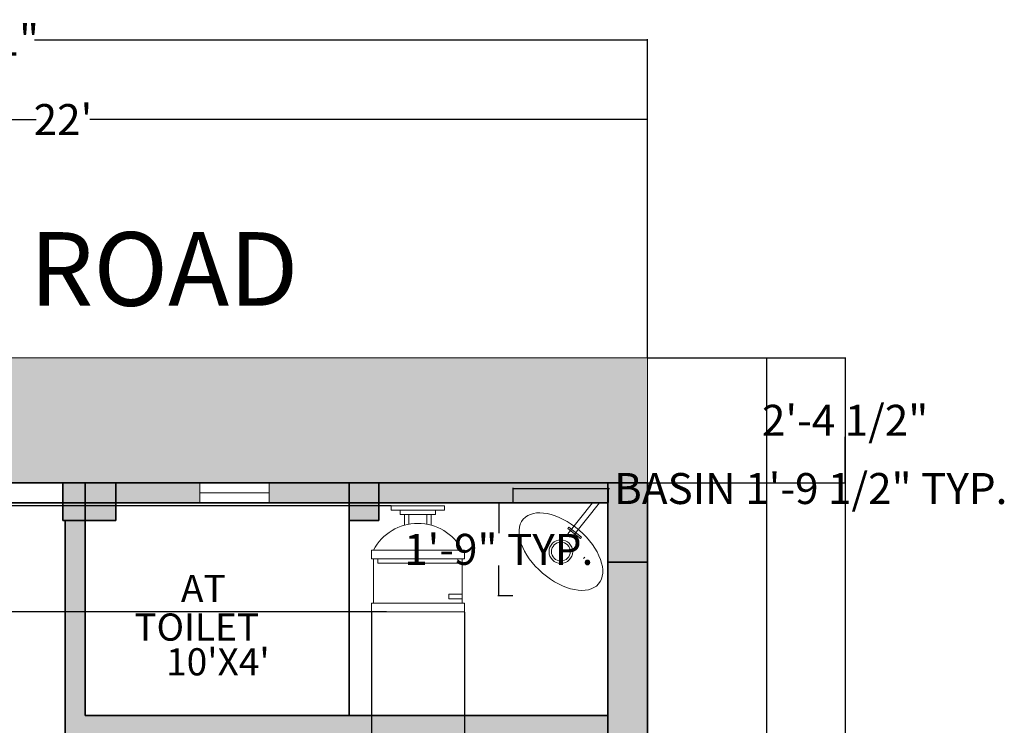
# Model space of a CAD drawing. Units: inches. Extents: x -17 to 892, y -721 to 172.
# Tile 11 of 11: x 655 to 877, y 7 to 166. Entities that reach past the tile are written whole.
import ezdxf

# ---------------------------------------------------------------- set-up
doc = ezdxf.new("R2010")
doc.units = ezdxf.units.IN
doc.header["$MEASUREMENT"] = 0
doc.layers.get('0').update_dxf_attribs({"color": 14})
for name, color, linetype, lineweight in [('A-ANNO-DIMS', 2, 'Continuous', 18), ('A-ANNO-TEXT', 7, 'Continuous', 18), ('A-AREA-IDEN', 7, 'Continuous', 18), ('A-COLS', 252, 'Continuous', 35), ('A-FLOR-FIXT', 8, 'Continuous', 18), ('A-WALL-PATT', 14, 'Continuous', 13), ('C-ROAD', 8, 'Continuous', 18), ('walls', 252, 'Continuous', 35), ('windows', 161, 'Continuous', 18)]:
    doc.layers.add(name, color=color, linetype=linetype, lineweight=lineweight)
doc.layers.add('A-COLS-PATT', color=254, linetype='Continuous', lineweight=13, true_color=0xd7ebd2)
doc.layers.add('C-ROAD-PATT', color=9, linetype='Continuous', lineweight=13, true_color=0xafd9aa)
doc.styles.get("Standard").update_dxf_attribs({"font": 'arial.ttf'})
doc.dimstyles.get("Standard").update_dxf_attribs({"dimtxt": 7, "dimasz": 0.18, "dimexe": 0.18, "dimexo": 0.0625, "dimgap": 0.09, "dimtad": 0, "dimtih": 1, "dimtoh": 1, "dimzin": 0, "dimdsep": 46, "dimlunit": 3, "dimtxsty": 'Standard', "dimcen": 0.09, "dimadec": 0, "dimazin": 0, "dimtfac": 1, "dimtofl": 0, "dimtmove": 0, "dimatfit": 3, "dimfxl": 1, "dimtolj": 1, "dimtzin": 0, "dimarcsym": 0})

# ---------------------------------------------------------------- blocks, each defined once
blk = doc.blocks.new('*U12')
for p, q in [((-10, 22), (-10, 12)), ((-10, 21), (-7, 21)), ((-7, 21), (-7, 20)), ((10, 12), (10, 22)), ((-7, 20), (-10, 20)), ((10.5, 12), (-10.5, 12)), ((-10.5, 10), (-10.5, 12)), ((9, 13), (-9, 13)), ((-9, 13), (-9, 12)), ((9, 12), (9, 13)), ((10.5, 12), (10.5, 10)), ((10.5, 10), (-10.5, 10)), ((-3, 4.4065), (-3, 2)), ((-2, 2), (-2, 4.1658)), ((2, 4.1658), (2, 2)), ((3, 2), (3, 4.4065)), ((4, 2), (-4, 2)), ((-4, 2), (-4, 1)), ((4, 1), (4, 2))]:
    blk.add_line(p, q)
for points in [[(10.5, 22), (10.5, 24), (-10.5, 24), (-10.5, 22)], [(6, 0), (6, 1), (-6, 1), (-6, 0)]]:
    blk.add_lwpolyline(points, close=True)
blk.add_arc((0, 15.3333), 11.3333, 208.0725, 331.9275)
blk = doc.blocks.new('*D17')
at = {"layer": 'A-ANNO-DIMS', "color": 0, "lineweight": -2, "transparency": 16777216}
for p, q in [((822.86, 89.9), (823.61, 89.9)), ((823.43, 89.72), (823.43, -263.08)), ((823.43, -623.21), (823.43, -270.41)), ((822.86, -623.39), (823.61, -623.39))]:
    blk.add_line(p, q, dxfattribs=at)
at = {"layer": 'A-ANNO-DIMS', "color": 0, "lineweight": 100, "transparency": 16777216}
for points in [[(823.4, 89.72), (823.46, 89.72), (823.43, 89.9)], [(823.4, -623.21), (823.46, -623.21), (823.43, -623.39)]]:
    blk.add_solid(points, dxfattribs=at)
at = {"layer": 'Defpoints', "color": 0, "lineweight": 100, "transparency": 16777216}
for p in [(822.8, 89.9), (822.8, -623.39), (823.43, -623.39)]:
    blk.add_point(p, dxfattribs=at)
at = {"layer": 'A-ANNO-DIMS', "color": 0, "transparency": 16777216, "insert": (823.43, -266.74), "char_height": 7, "attachment_point": 5}
blk.add_mtext('\\A1;57\'-1"', dxfattribs=at)
blk = doc.blocks.new('*D18')
at = {"layer": 'A-ANNO-DIMS', "color": 0, "lineweight": -2, "transparency": 16777216}
for p, q in [((532.58, 142.49), (532.58, 143.87)), ((532.76, 143.69), (658.49, 143.69)), ((796.4, 143.69), (670.67, 143.69)), ((796.58, 142.49), (796.58, 143.87))]:
    blk.add_line(p, q, dxfattribs=at)
at = {"layer": 'A-ANNO-DIMS', "color": 0, "lineweight": 100, "transparency": 16777216}
for points in [[(532.76, 143.72), (532.76, 143.66), (532.58, 143.69)], [(796.4, 143.72), (796.4, 143.66), (796.58, 143.69)]]:
    blk.add_solid(points, dxfattribs=at)
at = {"layer": 'Defpoints', "color": 0, "lineweight": 100, "transparency": 16777216}
for p in [(532.58, 142.43), (796.58, 143.69), (796.58, 142.43)]:
    blk.add_point(p, dxfattribs=at)
at = {"layer": 'A-ANNO-DIMS', "color": 0, "transparency": 16777216, "insert": (664.58, 143.69), "char_height": 7, "attachment_point": 5}
blk.add_mtext("\\A1;22'", dxfattribs=at)
blk = doc.blocks.new('BASIN-CORNER')
for p, q in [((11.05, 12.77), (16.6, 19.78)), ((18.18, 19.78), (12.02, 12)), ((11.25, 14.32), (11, 14)), ((11, 14), (13.87, 11.73)), ((14.12, 12.04), (11.25, 14.32)), ((12.02, 12), (11.05, 12.77)), ((13.87, 11.73), (14.12, 12.05))]:
    blk.add_line(p, q)
for radius in [2.67, 2.13, 2.13, 2.13]:
    blk.add_circle((9.46, 8.76), radius)
blk.add_ellipse((9.46, 8.76), major_axis=(-8.49, 7.31), ratio=0.56899)
blk = doc.blocks.new('*D48')
at = {"layer": 'A-ANNO-DIMS', "color": 0, "lineweight": -2, "transparency": 16777216}
for p, q in [((766.21, 57.17), (766.21, 60.53)), ((766.39, 60.35), (787.6, 60.35)), ((787.78, 57.17), (787.78, 60.53)), ((787.78, 60.35), (787.96, 60.35))]:
    blk.add_line(p, q, dxfattribs=at)
at = {"layer": 'A-ANNO-DIMS', "color": 0, "lineweight": 100, "transparency": 16777216}
for points in [[(766.39, 60.38), (766.39, 60.32), (766.21, 60.35)], [(787.6, 60.38), (787.6, 60.32), (787.78, 60.35)]]:
    blk.add_solid(points, dxfattribs=at)
at = {"layer": 'Defpoints', "color": 0, "lineweight": 100, "transparency": 16777216}
for p in [(787.78, 60.35), (766.21, 57.11), (787.78, 57.11)]:
    blk.add_point(p, dxfattribs=at)
at = {"layer": 'A-ANNO-DIMS', "color": 0, "transparency": 16777216, "insert": (833.42, 60.35), "char_height": 7, "attachment_point": 5}
blk.add_mtext('\\A1;BASIN 1\'-9 1/2" TYP.', dxfattribs=at)
blk = doc.blocks.new('*D49')
at = {"layer": 'A-ANNO-DIMS', "color": 0, "lineweight": -2, "transparency": 16777216}
for p, q in [((766.15, 57.11), (762.79, 57.11)), ((762.97, 56.93), (762.97, 50.28)), ((762.97, 36.3), (762.97, 42.95)), ((766.15, 36.12), (762.79, 36.12))]:
    blk.add_line(p, q, dxfattribs=at)
at = {"layer": 'A-ANNO-DIMS', "color": 0, "lineweight": 100, "transparency": 16777216}
for points in [[(762.94, 56.93), (763, 56.93), (762.97, 57.11)], [(762.94, 36.3), (763, 36.3), (762.97, 36.12)]]:
    blk.add_solid(points, dxfattribs=at)
at = {"layer": 'Defpoints', "color": 0, "lineweight": 100, "transparency": 16777216}
for p in [(762.97, 57.11), (766.21, 57.11), (766.21, 36.12)]:
    blk.add_point(p, dxfattribs=at)
at = {"layer": 'A-ANNO-DIMS', "color": 0, "transparency": 16777216, "insert": (762.97, 46.61), "char_height": 7, "attachment_point": 5}
blk.add_mtext('\\A1;1\'-9" TYP.', dxfattribs=at)
blk = doc.blocks.new('*D58')
at = {"layer": 'A-ANNO-DIMS', "color": 0, "lineweight": -2, "transparency": 16777216}
for p, q in [((495.38, 61.67), (495.38, 161.84)), ((495.56, 161.66), (633.81, 161.66)), ((796.4, 161.66), (658.15, 161.66)), ((796.58, 89.96), (796.58, 161.84))]:
    blk.add_line(p, q, dxfattribs=at)
at = {"layer": 'A-ANNO-DIMS', "color": 0, "lineweight": 100, "transparency": 16777216}
for points in [[(495.56, 161.69), (495.56, 161.63), (495.38, 161.66)], [(796.4, 161.69), (796.4, 161.63), (796.58, 161.66)]]:
    blk.add_solid(points, dxfattribs=at)
at = {"layer": 'Defpoints', "color": 0, "lineweight": 100, "transparency": 16777216}
for p in [(796.58, 161.66), (796.58, 89.9), (495.38, 61.61)]:
    blk.add_point(p, dxfattribs=at)
at = {"layer": 'A-ANNO-DIMS', "color": 0, "transparency": 16777216, "insert": (645.98, 161.66), "char_height": 7, "attachment_point": 5}
blk.add_mtext('\\A1;25\'-1"', dxfattribs=at)
blk = doc.blocks.new('*D59')
at = {"layer": 'A-ANNO-DIMS', "color": 0, "lineweight": -2, "transparency": 16777216}
for p, q in [((796.64, 89.9), (841.36, 89.9)), ((841.18, 89.72), (841.18, -281.05)), ((841.18, -659.16), (841.18, -288.38)), ((796.64, -659.34), (841.36, -659.34))]:
    blk.add_line(p, q, dxfattribs=at)
at = {"layer": 'A-ANNO-DIMS', "color": 0, "lineweight": 100, "transparency": 16777216}
for points in [[(841.15, 89.72), (841.21, 89.72), (841.18, 89.9)], [(841.15, -659.16), (841.21, -659.16), (841.18, -659.34)]]:
    blk.add_solid(points, dxfattribs=at)
at = {"layer": 'Defpoints', "color": 0, "lineweight": 100, "transparency": 16777216}
for p in [(796.58, 89.9), (841.18, 89.9), (796.58, -659.34)]:
    blk.add_point(p, dxfattribs=at)
at = {"layer": 'A-ANNO-DIMS', "color": 0, "transparency": 16777216, "insert": (841.18, -284.72), "char_height": 7, "attachment_point": 5}
blk.add_mtext('\\A1;62\'-5"', dxfattribs=at)
blk = doc.blocks.new('*D66')
at = {"layer": 'A-ANNO-DIMS', "color": 0, "lineweight": -2, "transparency": 16777216}
for p, q in [((796.64, 89.9), (841.36, 89.9)), ((841.18, 89.72), (841.18, 79.47)), ((841.18, 61.79), (841.18, 72.05)), ((796.64, 61.61), (841.36, 61.61))]:
    blk.add_line(p, q, dxfattribs=at)
at = {"layer": 'A-ANNO-DIMS', "color": 0, "lineweight": 100, "transparency": 16777216}
for points in [[(841.15, 89.72), (841.21, 89.72), (841.18, 89.9)], [(841.15, 61.79), (841.21, 61.79), (841.18, 61.61)]]:
    blk.add_solid(points, dxfattribs=at)
at = {"layer": 'Defpoints', "color": 0, "lineweight": 100, "transparency": 16777216}
for p in [(796.58, 89.9), (796.58, 61.61), (841.18, 61.61)]:
    blk.add_point(p, dxfattribs=at)
at = {"layer": 'A-ANNO-DIMS', "color": 0, "transparency": 16777216, "insert": (841.18, 75.76), "char_height": 7, "attachment_point": 5}
blk.add_mtext('\\A1;2\'-4 1/2"', dxfattribs=at)
blk = doc.blocks.new('*D67')
at = {"layer": 'A-ANNO-DIMS', "color": 0, "lineweight": -2, "transparency": 16777216}
for p, q in [((734.21, 32.4), (734.21, -704.12)), ((755.21, 32.4), (755.21, -704.12)), ((734.39, -703.94), (735.64, -703.94)), ((755.03, -703.94), (753.77, -703.94))]:
    blk.add_line(p, q, dxfattribs=at)
at = {"layer": 'A-ANNO-DIMS', "color": 0, "lineweight": 100, "transparency": 16777216}
for points in [[(734.39, -703.91), (734.39, -703.97), (734.21, -703.94)], [(755.03, -703.91), (755.03, -703.97), (755.21, -703.94)]]:
    blk.add_solid(points, dxfattribs=at)
at = {"layer": 'Defpoints', "color": 0, "lineweight": 100, "transparency": 16777216}
for p in [(734.21, 32.46), (755.21, 32.46), (755.21, -703.94)]:
    blk.add_point(p, dxfattribs=at)
at = {"layer": 'A-ANNO-DIMS', "color": 0, "transparency": 16777216, "insert": (744.71, -703.94), "char_height": 7, "attachment_point": 5}
blk.add_mtext('\\A1;1\'-9"', dxfattribs=at)
blk = doc.blocks.new('*D68')
at = {"layer": 'A-ANNO-DIMS', "color": 0, "lineweight": -2, "transparency": 16777216}
for p, q in [((738.65, 56.46), (1.11, 56.46)), ((1.29, 56.28), (1.29, 48.13)), ((1.29, 32.64), (1.29, 40.8)), ((737.65, 32.46), (1.11, 32.46))]:
    blk.add_line(p, q, dxfattribs=at)
at = {"layer": 'A-ANNO-DIMS', "color": 0, "lineweight": 100, "transparency": 16777216}
for points in [[(1.26, 56.28), (1.32, 56.28), (1.29, 56.46)], [(1.26, 32.64), (1.32, 32.64), (1.29, 32.46)]]:
    blk.add_solid(points, dxfattribs=at)
at = {"layer": 'Defpoints', "color": 0, "lineweight": 100, "transparency": 16777216}
for p in [(738.71, 56.46), (1.29, 32.46), (737.71, 32.46)]:
    blk.add_point(p, dxfattribs=at)
at = {"layer": 'A-ANNO-DIMS', "color": 0, "transparency": 16777216, "insert": (1.29, 44.46), "char_height": 7, "attachment_point": 5}
blk.add_mtext('\\A1;2\'-0"', dxfattribs=at)

msp = doc.modelspace()

# ---------------------------------------------------------------- hatches: boundary and pattern name
at = {"layer": 'A-COLS-PATT'}
h = msp.add_hatch(color=256, dxfattribs=at)
h.dxf.hatch_style = 1
h.paths.add_polyline_path([(92.084, -102.402), (83.084, -102.402), (83.084, -119.959), (92.084, -119.959)])
h.paths.add_polyline_path([(669.576, 61.611), (664.576, 61.611), (664.576, 57.111), (669.576, 57.111)])
h.paths.add_polyline_path([(676.541, 61.611), (669.576, 61.611), (669.576, 57.111), (676.541, 57.111)])
h.paths.add_polyline_path([(669.576, 57.111), (664.576, 57.111), (664.576, 53.097), (669.576, 53.097)])
h.paths.add_polyline_path([(676.541, 57.111), (669.576, 57.111), (669.576, 53.097), (676.541, 53.097)])
h.paths.add_polyline_path([(735.904, 61.611), (729.183, 61.611), (729.183, 57.111), (735.904, 57.111)])
h.paths.add_polyline_path([(735.904, 57.111), (729.183, 57.111), (729.183, 53.097), (735.904, 53.097)])
h = msp.add_hatch(color=256, dxfattribs=at)
h.dxf.hatch_style = 1
h.paths.add_polyline_path([(796.576, 61.611), (787.576, 61.611), (787.576, 43.692), (796.576, 43.692)])
h.paths.add_polyline_path([(796.576, -140.181), (787.576, -140.181), (787.576, -157.529), (796.576, -157.529)])
h.paths.add_polyline_path([(674.076, -107.889), (665.076, -107.889), (665.076, -116.615), (674.076, -116.615)])
h.paths.add_polyline_path([(537.076, -107.889), (532.576, -107.889), (532.576, -116.615), (537.076, -116.615)])
h.paths.add_polyline_path([(541.576, -207.597), (532.576, -207.597), (532.576, -223.04), (541.576, -223.04)])
h.paths.add_polyline_path([(541.576, -335.389), (532.576, -335.389), (532.576, -350.421), (541.576, -350.421)])
h.paths.add_polyline_path([(541.576, -412.049), (532.576, -412.049), (532.576, -420.971), (541.576, -420.971)])
h.paths.add_polyline_path([(674.076, -410.999), (665.076, -410.999), (665.076, -421.003), (674.076, -421.003)])
h.paths.add_polyline_path([(674.076, -329.432), (665.076, -329.432), (665.076, -335.389), (665.076, -343.822), (674.076, -343.822), (674.076, -335.389)])
h.paths.add_polyline_path([(667.076, -610.134), (659.076, -610.134), (659.076, -618.889), (659.101, -623.389), (667.076, -623.389)])
h.paths.add_polyline_path([(796.576, -610.134), (787.576, -610.134), (787.576, -614.389), (787.576, -623.342), (796.576, -623.342)])
h.paths.add_polyline_path([(796.576, -324.682), (787.576, -324.682), (787.576, -353.487), (796.576, -353.487)])
at = {"layer": 'A-WALL-PATT'}
h = msp.add_hatch(color=256, dxfattribs=at)
h.dxf.hatch_style = 1
h.paths.add_polyline_path([(669.576, 4.611), (787.576, 4.611), (787.576, 9.111), (669.576, 9.111), (669.576, 53.097), (665.076, 53.097), (665.076, -107.889), (669.576, -107.889)])
h.paths.add_polyline_path([(674.076, -116.615), (665.076, -116.615), (665.076, -154.389), (674.076, -154.389)])
h.paths.add_polyline_path([(787.576, -145.389), (713.344, -145.389), (713.344, -154.389), (787.576, -154.389)])
h.paths.add_polyline_path([(632.137, -145.389), (622.476, -145.389), (622.476, -154.389), (632.137, -154.389)])
h.paths.add_polyline_path([(554.583, -145.389), (537.076, -145.389), (537.076, -154.389), (554.583, -154.389)])
h.paths.add_polyline_path([(537.076, -145.389), (532.576, -145.389), (532.576, -154.389), (537.076, -154.389)])
h.paths.add_polyline_path([(537.076, -116.615), (532.576, -116.615), (532.576, -145.389), (537.076, -145.389)])
h.paths.add_polyline_path([(796.576, 43.692), (787.576, 43.692), (787.576, -140.181), (796.576, -140.181)])
h.paths.add_polyline_path([(541.576, -223.04), (532.576, -223.04), (532.576, -282.182), (537.076, -282.182), (541.576, -282.182)])
h.paths.add_polyline_path([(796.576, -157.529), (787.576, -157.529), (787.576, -324.682), (796.576, -324.682)])
h.paths.add_polyline_path([(554.583, -335.389), (541.576, -335.389), (541.576, -344.389), (554.583, -344.389)])
h.paths.add_polyline_path([(635.731, -335.389), (622.476, -335.389), (622.476, -344.389), (635.731, -344.389)])
h.paths.add_polyline_path([(541.576, -350.421), (532.576, -350.421), (532.576, -412.049), (541.576, -412.049)])
h.paths.add_polyline_path([(674.076, -343.822), (665.076, -343.822), (665.076, -410.999), (674.076, -410.999)])
h.paths.add_polyline_path([(667.076, -421.003), (665.076, -421.003), (659.076, -421.002), (659.076, -610.134), (667.076, -610.134)])
h.paths.add_polyline_path([(796.576, -353.487), (787.576, -353.487), (787.576, -610.134), (796.576, -610.134)])
h.paths.add_polyline_path([(787.576, -335.389), (775.362, -335.389), (775.362, -344.389), (787.576, -344.389)])
h.paths.add_polyline_path([(707.469, -335.389), (703.501, -335.389), (703.501, -344.389), (707.469, -344.389)])
h.paths.add_polyline_path([(695.494, 61.611), (676.541, 61.611), (676.541, 57.111), (695.494, 57.111)])
h.paths.add_polyline_path([(729.183, 61.611), (724.076, 61.611), (711.12, 61.611), (711.12, 57.111), (729.183, 57.111)])
h.paths.add_polyline_path([(787.576, 61.611), (735.904, 61.611), (735.904, 57.111), (787.576, 57.111)])
at = {"layer": 'C-ROAD-PATT'}
h = msp.add_hatch(dxfattribs=at)
h.set_pattern_fill('BRICK', color=256)
h.set_pattern_definition([(0, (449.49168, 0), (0, 0.25), []), (90, (449.4917, 0), (-0.5, 0), [0.25, -0.25]), (90, (449.7417, 0), (-0.5, 0), [-0.25, 0.25])])
h.paths.add_polyline_path([(796.576, 89.902), (532.576, 89.902), (532.576, 61.611), (796.576, 61.611)])

# ---------------------------------------------------------------- linework, layer by layer
at = {"layer": 'A-COLS'}
for p, q in [((664.576, 61.611), (664.576, 53.097)), ((676.541, 53.097), (676.541, 61.611)), ((729.183, 61.611), (729.183, 53.097)), ((735.904, 53.097), (735.904, 61.611)), ((664.576, 53.097), (676.541, 53.097)), ((729.183, 53.097), (735.904, 53.097)), ((787.576, 43.692), (796.576, 43.692))]:
    msp.add_line(p, q, dxfattribs=at)
at = {"layer": 'A-FLOR-FIXT'}
msp.add_line((782.13, 44.563), (782.38, 44.878), dxfattribs=at)
at = {"layer": 'C-ROAD'}
for p, q in [((532.576, 89.902), (796.576, 89.902)), ((796.576, 89.902), (796.576, 61.611))]:
    msp.add_line(p, q, dxfattribs=at)
at = {"layer": 'walls'}
for p, q in [((532.576, 61.611), (796.576, 61.611)), ((669.576, 9.111), (669.576, 61.611)), ((724.076, 61.611), (734.29, 61.611)), ((787.576, 61.611), (787.576, -614.389)), ((796.576, 61.611), (796.576, -623.389)), ((537.076, 57.111), (787.576, 57.111)), ((665.076, -107.889), (665.076, 53.097)), ((729.183, 53.097), (729.183, 9.111)), ((669.576, 9.111), (787.576, 9.111))]:
    msp.add_line(p, q, dxfattribs=at)
at = {"layer": 'windows'}
for p, q in [((695.494, 61.611), (695.494, 57.111)), ((695.494, 61.611), (695.494, 59.361)), ((711.12, 57.111), (711.12, 61.611)), ((695.494, 59.361), (711.12, 59.361))]:
    msp.add_line(p, q, dxfattribs=at)

# ---------------------------------------------------------------- block references
at = {"layer": 'A-FLOR-FIXT', "rotation": 180}
msp.add_blockref('*U12', (744.709, 56.461), dxfattribs=at)
at = {"layer": 'A-FLOR-FIXT'}
msp.add_blockref('BASIN-CORNER', (767.54, 37.333), dxfattribs=at)

# ---------------------------------------------------------------- texts
at = {"layer": 'A-ANNO-TEXT'}
msp.add_text('ROAD', height=16.6398, dxfattribs=at).set_placement((657.053, 101.621))
at = {"layer": 'A-AREA-IDEN'}
for s, p in [('AT', (691.207, 34.704)), ('TOILET', (680.695, 25.988)), ("10'X4'", (687.862, 18.136))]:
    msp.add_text(s, height=6.1361, dxfattribs=at).set_placement(p)

# ---------------------------------------------------------------- dimensions: what is measured, and where the dimension line sits
at = {"layer": 'A-ANNO-DIMS'}
for base, p1, p2, override, picture, middle in [((796.576, 161.663), (495.384, 61.611), (796.576, 89.902), {"dimdec": 1, "dimlfac": 1, "dimrnd": 0, "dimzin": 1, "dimdsep": 46, "dimlunit": 4, "dimfrac": 2}, '*D58', (645.98, 161.663)), ((796.576, 143.692), (532.576, 142.427), (796.576, 142.427), {"dimclrd": 0, "dimclre": 0, "dimclrt": 0}, '*D18', (664.576, 143.692)), ((755.209, -703.936), (734.209, 32.461), (755.209, 32.461), {"dimdec": 1, "dimlfac": 1, "dimrnd": 0, "dimzin": 1, "dimdsep": 46, "dimlunit": 4, "dimfrac": 2}, '*D67', (744.709, -703.936))]:
    dim = msp.add_linear_dim(base=base, p1=p1, p2=p2, dimstyle='Standard', override=override, dxfattribs=at)
    dim.commit()
    dim.dimension.update_dxf_attribs({"geometry": picture, "text_midpoint": middle})
for base, p1, p2, picture, middle in [((841.176, 89.902), (796.576, -659.336), (796.576, 89.902), '*D59', (841.176, -284.717)), ((841.176, 61.611), (796.576, 89.902), (796.576, 61.611), '*D66', (841.176, 75.756)), ((1.292, 32.461), (738.709, 56.461), (737.709, 32.461), '*D68', (1.292, 44.461))]:
    dim = msp.add_linear_dim(base=base, p1=p1, p2=p2, angle=90, dimstyle='Standard', override={"dimdec": 1, "dimlfac": 1, "dimrnd": 0, "dimzin": 1, "dimdsep": 46, "dimlunit": 4, "dimfrac": 2}, dxfattribs=at)
    dim.commit()
    dim.dimension.update_dxf_attribs({"geometry": picture, "text_midpoint": middle})
for base, p1, p2, text, override, picture, middle in [((823.427, -623.389), (822.802, 89.902), (822.802, -623.389), '57\'-1"', {"dimclrd": 0, "dimclre": 0, "dimclrt": 0}, '*D17', (823.427, -266.744)), ((762.973, 57.111), (766.209, 36.117), (766.209, 57.111), '<> TYP.', {"dimdec": 1, "dimlfac": 1, "dimrnd": 0, "dimzin": 1, "dimdsep": 46, "dimlunit": 4, "dimfrac": 2}, '*D49', (762.973, 46.614))]:
    dim = msp.add_linear_dim(base=base, p1=p1, p2=p2, angle=90, text=text, dimstyle='Standard', override=override, dxfattribs=at)
    dim.commit()
    dim.dimension.update_dxf_attribs({"geometry": picture, "text_midpoint": middle})
dim = msp.add_linear_dim(base=(787.781, 60.347), p1=(766.209, 57.111), p2=(787.781, 57.111), text='BASIN <> TYP.', dimstyle='Standard', override={"dimdec": 1, "dimlfac": 1, "dimrnd": 0, "dimzin": 1, "dimdsep": 46, "dimlunit": 4, "dimfrac": 2}, dxfattribs=at)
dim.commit()
dim.dimension.update_dxf_attribs({"geometry": '*D48', "text_midpoint": (833.418, 60.347)})

doc.saveas('drawing.dxf')
